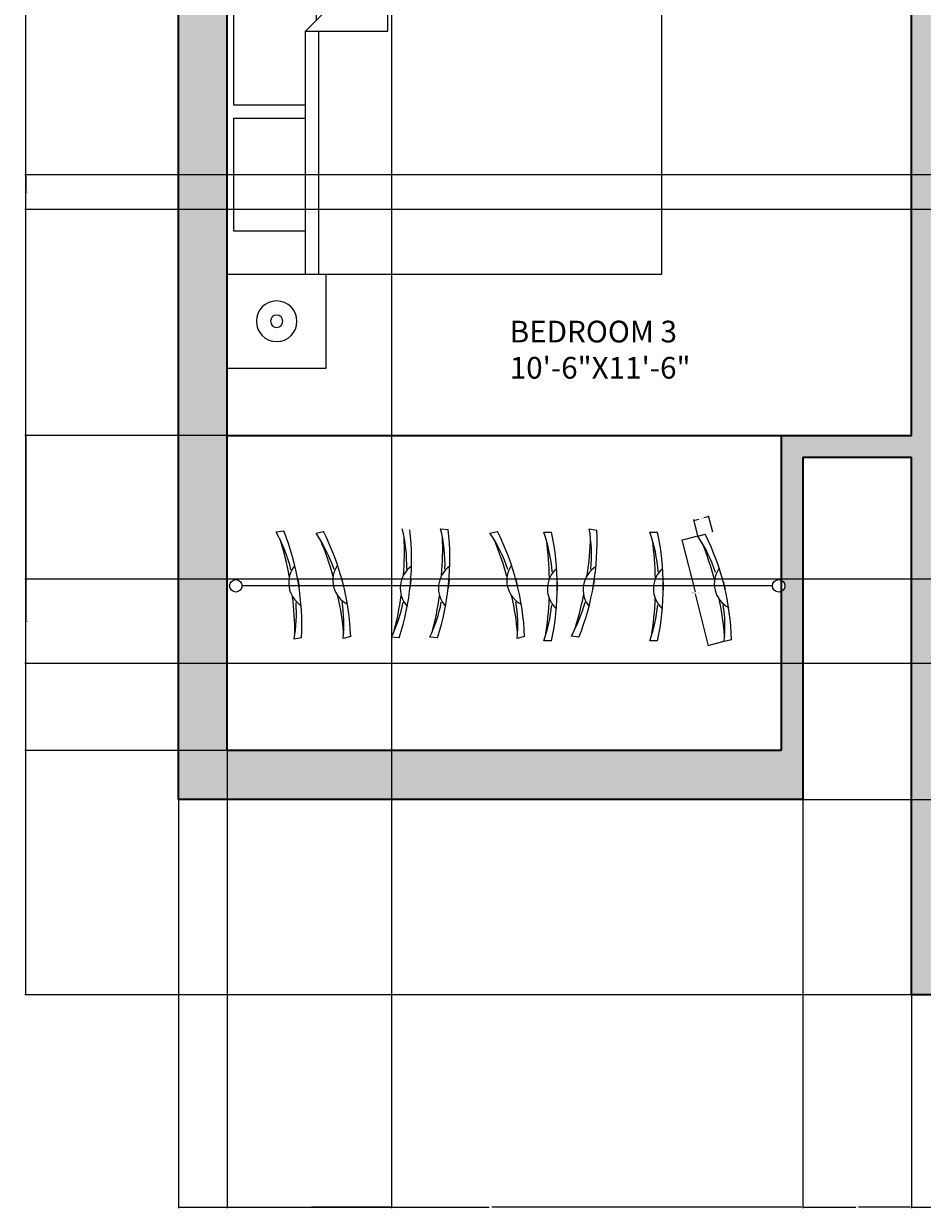
# Model space of a CAD drawing. Units: inches. Extents: x -29 to 443, y -589 to 39.
# Tile 1 of 5: x -29 to 136, y -493 to -275. Entities that reach past the tile are written whole.
import ezdxf

# ---------------------------------------------------------------- set-up
doc = ezdxf.new("R2010")
doc.units = ezdxf.units.IN
for name, color, linetype, lineweight in [('A-ANNO-DIMS', 2, 'Continuous', 18), ('A-AREA-IDEN', 7, 'Continuous', 18), ('A-FLOR-CASE', 8, 'Continuous', 18), ('A-FURN', 9, 'Continuous', 18), ('A-WALL', 7, 'Continuous', 35)]:
    doc.layers.add(name, color=color, linetype=linetype, lineweight=lineweight)
doc.layers.add('A-WALL-PATT', color=251, linetype='Continuous', lineweight=13, true_color=0x636466)
doc.styles.get("Standard").update_dxf_attribs({"font": 'arial.ttf'})
doc.dimstyles.get("Standard").update_dxf_attribs({"dimtxt": 0.18, "dimasz": 0.18, "dimexe": 0.18, "dimexo": 0.0625, "dimgap": 0.09, "dimtad": 0, "dimtih": 1, "dimtoh": 1, "dimdec": 4, "dimzin": 0, "dimdsep": 46, "dimtxsty": 'Standard', "dimcen": 0.09, "dimadec": 0, "dimazin": 0, "dimtfac": 1, "dimtdec": 4, "dimtofl": 0, "dimtmove": 0, "dimatfit": 3, "dimfxl": 1, "dimtolj": 1, "dimtzin": 0, "dimarcsym": 0})

# ---------------------------------------------------------------- blocks, each defined once
blk = doc.blocks.new('Bed - Queen')
for p, q in [((0, -80.00003), (0, 0)), ((0, 0), (59.99999, 0)), ((59.99999, 0), (59.99999, -80.00003)), ((7.99999, -1.2), (28.79998, -1.2)), ((7.99999, -14.4), (7.99999, -1.2)), ((28.79998, -1.2), (28.79998, -14.4)), ((31.19999, -1.2), (51.99999, -1.2)), ((31.19999, -14.4), (31.19999, -1.2)), ((51.99999, -1.2), (51.99999, -16.4)), ((0, -14.4), (44.8, -14.4)), ((59.99999, -29.6), (44.8, -14.4)), ((44.8, -14.4), (44.8, -29.6)), ((44.8, -16.8), (0, -16.8)), ((51.99999, -16.4), (46.79936, -16.4)), ((44.8, -29.6), (59.99999, -29.6)), ((59.99999, -80.00003), (0, -80.00003))]:
    blk.add_line(p, q)
blk = doc.blocks.new('NIGHTSTAND-SMALL')
blk.add_lwpolyline([(18.21, 17.2), (18.21, 0), (0, 0), (0, 17.2)], close=True)
for radius in [3.74, 1.13]:
    blk.add_circle((9.11, 8.6), radius)
blk = doc.blocks.new('CLOSET-HANGER')
for p, q in [((0, 20), (1.41, 20)), ((2.48, 10.82), (2.48, 9.31)), ((1.41, 0), (0, 0))]:
    blk.add_line(p, q)
for centre, radius, start, end in [((-25.67, 10.78), 27.27, 4.0274, 19.7451), ((-44.73, 10), 47.21, 347.7725, 12.2275), ((-51.84, 10.97), 52.87, 0.586, 8.2931), ((5.62, 9.59), 4.96, 130.682, 228.431), ((-25.8, 9.2), 27.39, 340.3791, 354.5177), ((-51.82, 9.48), 52.84, 350.6368, 358.15)]:
    blk.add_arc(centre, radius, start, end)
blk = doc.blocks.new('*D16')
at = {"layer": 'A-ANNO-DIMS', "color": 0, "lineweight": -2, "transparency": 16777216}
for p, q in [((95.05, -369.15), (92.03, -369.91)), ((92.24, -370.04), (94.58, -379.38)), ((97, -389.09), (94.67, -379.75)), ((99.9, -388.55), (96.87, -389.31))]:
    blk.add_line(p, q, dxfattribs=at)
at = {"layer": 'A-ANNO-DIMS', "color": 0, "transparency": 16777216}
for points in [[(92.27, -370.03), (92.21, -370.05), (92.2, -369.86)], [(97.03, -389.08), (96.97, -389.1), (97.05, -389.26)]]:
    blk.add_solid(points, dxfattribs=at)
at = {"layer": 'Defpoints', "color": 0, "transparency": 16777216}
for p in [(92.2, -369.86), (95.11, -369.14), (99.96, -388.54)]:
    blk.add_point(p, dxfattribs=at)
at = {"layer": 'A-ANNO-DIMS', "color": 0, "transparency": 16777216, "insert": (94.62, -379.56), "char_height": 0.18, "attachment_point": 5}
blk.add_mtext('\\A1;HANGER 20 TYP.', dxfattribs=at)
blk = doc.blocks.new('*D17')
at = {"layer": 'A-ANNO-DIMS', "color": 0, "lineweight": -2, "transparency": 16777216}
for p, q in [((95.09, -369.08), (94.34, -366.05)), ((94.56, -366.18), (95.3, -366)), ((96.96, -365.58), (96.22, -365.77)), ((97.85, -368.39), (97.09, -365.37))]:
    blk.add_line(p, q, dxfattribs=at)
at = {"layer": 'A-ANNO-DIMS', "color": 0, "transparency": 16777216}
for points in [[(94.55, -366.15), (94.57, -366.21), (94.38, -366.23)], [(96.95, -365.55), (96.97, -365.61), (97.14, -365.54)]]:
    blk.add_solid(points, dxfattribs=at)
at = {"layer": 'Defpoints', "color": 0, "transparency": 16777216}
for p in [(97.14, -365.54), (97.86, -368.45), (95.11, -369.14)]:
    blk.add_point(p, dxfattribs=at)
at = {"layer": 'A-ANNO-DIMS', "color": 0, "transparency": 16777216, "insert": (95.76, -365.88), "char_height": 0.18, "attachment_point": 5}
blk.add_mtext('\\A1;3 TYP.', dxfattribs=at)
blk = doc.blocks.new('*D37')
at = {"layer": 'A-ANNO-DIMS', "color": 0, "lineweight": -2, "transparency": 16777216}
for p, q in [((-0.63, 14.39), (-28.85, 14.39)), ((-28.67, 14.21), (-28.67, -219.43)), ((-28.67, -453.43), (-28.67, -219.8)), ((134.37, -453.61), (-28.85, -453.61))]:
    blk.add_line(p, q, dxfattribs=at)
at = {"layer": 'A-ANNO-DIMS', "color": 0, "transparency": 16777216}
for points in [[(-28.7, 14.21), (-28.64, 14.21), (-28.67, 14.39)], [(-28.7, -453.43), (-28.64, -453.43), (-28.67, -453.61)]]:
    blk.add_solid(points, dxfattribs=at)
at = {"layer": 'Defpoints', "color": 0, "transparency": 16777216}
for p in [(-0.56, 14.39), (-28.67, -453.61), (134.44, -453.61)]:
    blk.add_point(p, dxfattribs=at)
at = {"layer": 'A-ANNO-DIMS', "color": 0, "transparency": 16777216, "insert": (-28.67, -219.61), "char_height": 0.18, "attachment_point": 5}
blk.add_mtext('\\A1;468', dxfattribs=at)
blk = doc.blocks.new('*D38')
at = {"layer": 'A-ANNO-DIMS', "color": 0, "lineweight": -2, "transparency": 16777216}
for p, q in [((8.44, 5.32), (8.44, -492.89)), ((38.66, 5.51), (38.66, -492.89)), ((8.62, -492.71), (23.16, -492.71)), ((38.48, -492.71), (23.94, -492.71))]:
    blk.add_line(p, q, dxfattribs=at)
at = {"layer": 'A-ANNO-DIMS', "color": 0, "transparency": 16777216}
for points in [[(8.62, -492.68), (8.62, -492.74), (8.44, -492.71)], [(38.48, -492.68), (38.48, -492.74), (38.66, -492.71)]]:
    blk.add_solid(points, dxfattribs=at)
at = {"layer": 'Defpoints', "color": 0, "transparency": 16777216}
for p in [(8.44, 5.39), (38.66, 5.58), (8.44, -492.71)]:
    blk.add_point(p, dxfattribs=at)
at = {"layer": 'A-ANNO-DIMS', "color": 0, "transparency": 16777216, "insert": (23.55, -492.71), "char_height": 0.18, "attachment_point": 5}
blk.add_mtext('\\A1;30.23', dxfattribs=at)
blk = doc.blocks.new('*D42')
at = {"layer": 'A-ANNO-DIMS', "color": 0, "lineweight": -2, "transparency": 16777216}
for p, q in [((114.5, -417.61), (383.85, -417.61)), ((383.67, -417.79), (383.67, -435.43)), ((383.67, -453.43), (383.67, -435.8)), ((134.5, -453.61), (383.85, -453.61))]:
    blk.add_line(p, q, dxfattribs=at)
at = {"layer": 'A-ANNO-DIMS', "color": 0, "transparency": 16777216}
for points in [[(383.64, -417.79), (383.7, -417.79), (383.67, -417.61)], [(383.64, -453.43), (383.7, -453.43), (383.67, -453.61)]]:
    blk.add_solid(points, dxfattribs=at)
at = {"layer": 'Defpoints', "color": 0, "transparency": 16777216}
for p in [(114.44, -417.61), (134.44, -453.61), (383.67, -453.61)]:
    blk.add_point(p, dxfattribs=at)
at = {"layer": 'A-ANNO-DIMS', "color": 0, "transparency": 16777216, "insert": (383.67, -435.61), "char_height": 0.18, "attachment_point": 5}
blk.add_mtext('\\A1;36', dxfattribs=at)
blk = doc.blocks.new('*D46')
at = {"layer": 'A-ANNO-DIMS', "color": 0, "lineweight": -2, "transparency": 16777216}
for p, q in [((114.44, -417.68), (114.44, -492.89)), ((134.44, -453.68), (134.44, -492.89)), ((114.62, -492.71), (124.22, -492.71)), ((134.26, -492.71), (124.66, -492.71))]:
    blk.add_line(p, q, dxfattribs=at)
at = {"layer": 'A-ANNO-DIMS', "color": 0, "transparency": 16777216}
for points in [[(114.62, -492.68), (114.62, -492.74), (114.44, -492.71)], [(134.26, -492.68), (134.26, -492.74), (134.44, -492.71)]]:
    blk.add_solid(points, dxfattribs=at)
at = {"layer": 'Defpoints', "color": 0, "transparency": 16777216}
for p in [(114.44, -417.61), (134.44, -453.61), (134.44, -492.71)]:
    blk.add_point(p, dxfattribs=at)
at = {"layer": 'A-ANNO-DIMS', "color": 0, "transparency": 16777216, "insert": (124.44, -492.71), "char_height": 0.18, "attachment_point": 5}
blk.add_mtext('\\A1;20', dxfattribs=at)
blk = doc.blocks.new('*D47')
at = {"layer": 'A-ANNO-DIMS', "color": 0, "lineweight": -2, "transparency": 16777216}
for p, q in [((-0.56, -417.68), (-0.56, -492.89)), ((114.44, -417.68), (114.44, -492.89)), ((-0.38, -492.71), (56.65, -492.71)), ((114.26, -492.71), (57.22, -492.71))]:
    blk.add_line(p, q, dxfattribs=at)
at = {"layer": 'A-ANNO-DIMS', "color": 0, "transparency": 16777216}
for points in [[(-0.38, -492.68), (-0.38, -492.74), (-0.56, -492.71)], [(114.26, -492.68), (114.26, -492.74), (114.44, -492.71)]]:
    blk.add_solid(points, dxfattribs=at)
at = {"layer": 'Defpoints', "color": 0, "transparency": 16777216}
for p in [(-0.56, -417.61), (114.44, -417.61), (114.44, -492.71)]:
    blk.add_point(p, dxfattribs=at)
at = {"layer": 'A-ANNO-DIMS', "color": 0, "transparency": 16777216, "insert": (56.94, -492.71), "char_height": 0.18, "attachment_point": 5}
blk.add_mtext('\\A1;115', dxfattribs=at)
blk = doc.blocks.new('*D48')
at = {"layer": 'A-ANNO-DIMS', "color": 0, "lineweight": -2, "transparency": 16777216}
for p, q in [((110.37, -350.61), (-28.85, -350.61)), ((-28.67, -350.79), (-28.67, -379.43)), ((-28.67, -408.43), (-28.67, -379.8)), ((110.37, -408.61), (-28.85, -408.61))]:
    blk.add_line(p, q, dxfattribs=at)
at = {"layer": 'A-ANNO-DIMS', "color": 0, "transparency": 16777216}
for points in [[(-28.7, -350.79), (-28.64, -350.79), (-28.67, -350.61)], [(-28.7, -408.43), (-28.64, -408.43), (-28.67, -408.61)]]:
    blk.add_solid(points, dxfattribs=at)
at = {"layer": 'Defpoints', "color": 0, "transparency": 16777216}
for p in [(-28.67, -350.61), (110.44, -350.61), (110.44, -408.61)]:
    blk.add_point(p, dxfattribs=at)
at = {"layer": 'A-ANNO-DIMS', "color": 0, "transparency": 16777216, "insert": (-28.67, -379.61), "char_height": 0.18, "attachment_point": 5}
blk.add_mtext('\\A1;58', dxfattribs=at)
blk = doc.blocks.new('*D54')
at = {"layer": 'A-ANNO-DIMS', "color": 0, "lineweight": -2, "transparency": 16777216}
for p, q in [((134.44, -453.68), (134.44, -492.89)), ((147.44, -453.68), (147.44, -492.89)), ((134.62, -492.71), (140.73, -492.71)), ((147.26, -492.71), (141.15, -492.71))]:
    blk.add_line(p, q, dxfattribs=at)
at = {"layer": 'A-ANNO-DIMS', "color": 0, "transparency": 16777216}
for points in [[(134.62, -492.68), (134.62, -492.74), (134.44, -492.71)], [(147.26, -492.68), (147.26, -492.74), (147.44, -492.71)]]:
    blk.add_solid(points, dxfattribs=at)
at = {"layer": 'Defpoints', "color": 0, "transparency": 16777216}
for p in [(134.44, -453.61), (147.44, -453.61), (147.44, -492.71)]:
    blk.add_point(p, dxfattribs=at)
at = {"layer": 'A-ANNO-DIMS', "color": 0, "transparency": 16777216, "insert": (140.94, -492.71), "char_height": 0.18, "attachment_point": 5}
blk.add_mtext('\\A1;13', dxfattribs=at)
blk = doc.blocks.new('*D84')
at = {"layer": 'A-ANNO-DIMS', "color": 0, "lineweight": -2, "transparency": 16777216}
for p, q in [((350.37, -302.61), (-28.85, -302.61)), ((-28.67, -302.79), (-28.67, -305.61)), ((-28.67, -308.79), (-28.67, -305.97)), ((347.03, -308.97), (-28.85, -308.97))]:
    blk.add_line(p, q, dxfattribs=at)
at = {"layer": 'A-ANNO-DIMS', "color": 0, "transparency": 16777216}
for points in [[(-28.7, -302.79), (-28.64, -302.79), (-28.67, -302.61)], [(-28.7, -308.79), (-28.64, -308.79), (-28.67, -308.97)]]:
    blk.add_solid(points, dxfattribs=at)
at = {"layer": 'Defpoints', "color": 0, "transparency": 16777216}
for p in [(350.44, -302.61), (-28.67, -308.97), (347.09, -308.97)]:
    blk.add_point(p, dxfattribs=at)
at = {"layer": 'A-ANNO-DIMS', "color": 0, "transparency": 16777216, "insert": (-28.67, -305.79), "char_height": 0.18, "attachment_point": 5}
blk.add_mtext('\\A1;6.353', dxfattribs=at)
blk = doc.blocks.new('*D85')
at = {"layer": 'A-ANNO-DIMS', "color": 0, "lineweight": -2, "transparency": 16777216}
for p, q in [((346.2, -377.07), (-28.85, -377.07)), ((-28.67, -377.25), (-28.67, -384.66)), ((-28.67, -392.43), (-28.67, -385.02)), ((350.37, -392.61), (-28.85, -392.61))]:
    blk.add_line(p, q, dxfattribs=at)
at = {"layer": 'A-ANNO-DIMS', "color": 0, "transparency": 16777216}
for points in [[(-28.7, -377.25), (-28.64, -377.25), (-28.67, -377.07)], [(-28.7, -392.43), (-28.64, -392.43), (-28.67, -392.61)]]:
    blk.add_solid(points, dxfattribs=at)
at = {"layer": 'Defpoints', "color": 0, "transparency": 16777216}
for p in [(-28.67, -377.07), (346.26, -377.07), (350.44, -392.61)]:
    blk.add_point(p, dxfattribs=at)
at = {"layer": 'A-ANNO-DIMS', "color": 0, "transparency": 16777216, "insert": (-28.67, -384.84), "char_height": 0.18, "attachment_point": 5}
blk.add_mtext('\\A1;15.544', dxfattribs=at)

msp = doc.modelspace()

# ---------------------------------------------------------------- hatches: boundary and pattern name
at = {"layer": 'A-WALL-PATT'}
h = msp.add_hatch(color=256, dxfattribs=at)
h.dxf.hatch_style = 1
h.paths.add_polyline_path([(8.4359, 5.3851), (38.6638, 5.3851), (38.6638, 14.3851), (-0.5641, 14.3851), (-0.5641, -161.7206), (8.4359, -161.7206), (8.4359, -154.6149), (98.4359, -154.6149), (98.4359, -169.6149), (102.4359, -169.6149), (102.4359, -154.6149), (144.4359, -154.6149), (144.4359, -141.6149), (140.4359, -141.6149), (140.4359, -150.6149), (8.4359, -150.6149)])
h.paths.add_polyline_path([(153.762, 14.3851), (92.6638, 14.3851), (92.6638, 5.3851), (140.4359, 5.3851), (140.4359, -105.5868), (144.4359, -105.5868), (144.4359, -94.6149), (153.4359, -94.6149), (153.4359, -90.6149), (144.4359, -90.6149), (144.4359, 5.3851), (153.762, 5.3851)])
h.paths.add_polyline_path([(264.576, 14.3851), (189.762, 14.3851), (189.762, 5.3851), (204.4359, 5.3851), (204.4359, -40.0486, -0.11439146), (204.5889, -40.7086), (204.5889, -67.7086, -0.11439146), (204.4359, -68.3685), (204.4359, -90.6149), (183.4359, -90.6149), (183.4359, -94.6149), (204.4359, -94.6149), (204.4359, -108.4622), (208.4359, -108.4622), (208.4359, 5.3851), (264.576, 5.3851)])
h.paths.add_polyline_path([(359.4359, 14.3851), (318.576, 14.3851), (318.576, 5.3851), (350.4359, 5.3851), (350.4359, -150.6149), (208.4359, -150.6149), (208.4359, -144.6149), (204.4359, -144.6149), (204.4359, -154.6149), (286.4359, -154.6149), (286.4359, -169.4775), (290.4359, -169.4775), (290.4359, -154.6149), (359.4359, -154.6149)])
h.paths.add_polyline_path([(8.4359, -212.6149), (98.4359, -212.6149), (102.4359, -212.6149), (102.4359, -199.6149), (98.4359, -199.6149), (98.4359, -208.6149), (8.4359, -208.6149), (8.4359, -197.7206), (-0.5641, -197.7206), (-0.5641, -417.6149), (114.4359, -417.6149), (114.4359, -354.6149), (134.4359, -354.6149), (134.4359, -453.6149), (147.4359, -453.6149), (147.4359, -444.6149), (138.4359, -444.6149), (138.4359, -212.6149), (129.4359, -212.6149), (129.4359, -216.6149), (134.4359, -216.6149), (134.4359, -350.6149), (110.4359, -350.6149), (110.4359, -377.2063, -0.30395766), (111.1497, -378.2719, -0.30395766), (110.4359, -379.3376), (110.4359, -408.6149), (8.4359, -408.6149)])
h.paths.add_polyline_path([(265.0252, -444.6149), (230.4359, -444.6149), (230.4359, -396.6149), (246.223, -396.6149), (246.223, -392.6149), (230.4359, -392.6149), (230.4359, -302.6149), (245.4886, -302.6149), (245.4886, -298.6149), (226.4359, -298.6149), (226.4359, -444.6149), (189.4359, -444.6149), (189.4359, -453.6149), (226.4359, -453.6149), (265.0252, -453.6149)])
h.paths.add_polyline_path([(359.4359, -417.6149), (359.4359, -377.3771), (350.4359, -377.3771), (350.4359, -392.6149), (276.3235, -392.6149), (276.3235, -396.6149), (350.4359, -396.6149), (350.4359, -408.6149), (350.4359, -444.6149), (319.0252, -444.6149), (319.0252, -453.6149), (359.4359, -453.6149)])
h.paths.add_polyline_path([(359.4359, -298.6149), (290.4359, -298.6149), (290.4359, -289.6207), (286.4359, -289.6207), (286.4359, -298.6149), (277.8355, -298.6149), (277.8355, -302.6149), (350.4359, -302.6149), (350.4359, -323.3771), (359.4359, -323.3771)])
h.paths.add_polyline_path([(290.4359, -226.7916), (286.4359, -226.7916), (286.4359, -253.468), (290.4359, -253.468)])

# ---------------------------------------------------------------- linework, layer by layer
at = {"layer": 'A-FLOR-CASE'}
msp.add_line((108.8451, -378.2885), (11.1271, -378.2885), dxfattribs=at)
for centre in [(10.0136, -378.2719), (109.9973, -378.2719)]:
    msp.add_circle(centre, 1.1524, dxfattribs=at)
at = {"layer": 'A-FURN'}
for p, q in [((42.2396, -377.1753), (42.0915, -378.6789)), ((40.1179, -387.8399), (38.7157, -387.7018))]:
    msp.add_line(p, q, dxfattribs=at)
for centre, radius, start, end in [((-4.8169, -373.367), 47.208, 342.146968, 6.602004), ((14.2251, -374.4549), 27.2748, 358.401871, 14.119601), ((-11.8003, -371.7039), 52.8739, 354.960525, 2.667625), ((45.2498, -378.7105), 4.9606, 125.05649, 222.805441), ((13.9423, -376.0198), 27.3896, 334.753545, 348.892145), ((-11.9296, -373.1867), 52.8401, 345.011307, 352.524443)]:
    msp.add_arc(centre, radius, start, end, dxfattribs=at)
at = {"layer": 'A-WALL'}
for p, q in [((-0.5641, -417.6149), (-0.5641, 14.3851)), ((8.4359, -408.6149), (8.4359, -212.6149)), ((134.4359, -350.6149), (134.4359, -216.6149)), ((8.4359, -350.6149), (134.4359, -350.6149)), ((110.4359, -350.6149), (110.4359, -408.6149)), ((114.4359, -354.6149), (114.4359, -417.6149)), ((114.4359, -354.6149), (134.4359, -354.6149)), ((134.4359, -453.6149), (134.4359, -354.6149)), ((110.4359, -408.6149), (8.4359, -408.6149)), ((114.4359, -417.6149), (-0.5641, -417.6149)), ((147.4359, -453.6149), (134.4359, -453.6149))]:
    msp.add_line(p, q, dxfattribs=at)

# ---------------------------------------------------------------- block references
at = {"layer": 'A-FURN'}
for name, p, rotation in [('Bed - Queen', (8.4359, -320.9746), 90), ('CLOSET-HANGER', (20.7428, -388.0921), 9.453816115787394), ('CLOSET-HANGER', (29.8103, -387.9607), 14.5215371830677), ('CLOSET-HANGER', (45.7603, -387.7013), 354.3744866708974), ('CLOSET-HANGER', (61.8318, -387.9607), 14.52153718384618), ('CLOSET-HANGER', (71.8123, -387.5212), 350.5462235724349), ('CLOSET-HANGER', (99.9555, -388.5376), 14.02384461538142)]:
    msp.add_blockref(name, p, dxfattribs=dict(at, rotation=rotation))
at = {"layer": 'A-FURN', "extrusion": (0, 0, -1), "zscale": -1}
msp.add_blockref('NIGHTSTAND-SMALL', (-26.6499, -338.1702), dxfattribs=at)
at = {"layer": 'A-FURN'}
for p in [(66.7362, -388.403), (86.259, -388.403)]:
    msp.add_blockref('CLOSET-HANGER', p, dxfattribs=at)

# ---------------------------------------------------------------- texts
at = {"layer": 'A-AREA-IDEN', "insert": (60.4633, -329.4633), "char_height": 4, "attachment_point": 1}
msp.add_mtext_dynamic_manual_height_columns('BEDROOM 3\\P10\'-6"X11\'-6"', width=60.26419, gutter_width=12.5, heights=[0], dxfattribs=at)

# ---------------------------------------------------------------- dimensions: what is measured, and where the dimension line sits
at = {"layer": 'A-ANNO-DIMS'}
for base, p1, p2, override, picture, middle in [((-28.6698, -453.6149), (-0.5641, 14.3851), (134.4359, -453.6149), {"dimdec": 0, "dimlfac": 1, "dimrnd": 0, "dimzin": 0, "dimdsep": 46, "dimlunit": 2}, '*D37', (-28.6698, -219.6149)), ((-28.6698, -308.9679), (350.4359, -302.6149), (347.093, -308.9679), {"dimdec": 3, "dimlfac": 1, "dimrnd": 0, "dimzin": 0, "dimdsep": 46, "dimlunit": 2}, '*D84', (-28.6698, -305.7914)), ((-28.6698, -350.6149), (110.4359, -408.6149), (110.4359, -350.6149), {"dimdec": 0, "dimlfac": 1, "dimrnd": 0, "dimzin": 0, "dimdsep": 46, "dimlunit": 2}, '*D48', (-28.6698, -379.6149)), ((-28.6698, -377.0712), (350.4359, -392.6149), (346.2626, -377.0712), {"dimdec": 3, "dimlfac": 1, "dimrnd": 0, "dimzin": 0, "dimdsep": 46, "dimlunit": 2}, '*D85', (-28.6698, -384.8431)), ((383.6659, -453.6149), (114.4359, -417.6149), (134.4359, -453.6149), {"dimdec": 0, "dimlfac": 1, "dimrnd": 0, "dimzin": 0, "dimdsep": 46, "dimlunit": 2}, '*D42', (383.6659, -435.6149))]:
    dim = msp.add_linear_dim(base=base, p1=p1, p2=p2, angle=90, dimstyle='Standard', override=override, dxfattribs=at)
    dim.commit()
    dim.dimension.update_dxf_attribs({"geometry": picture, "text_midpoint": middle})
for base, p1, p2, override, picture, middle in [((8.4359, -492.7145), (38.6638, 5.5764), (8.4359, 5.3851), {"dimdec": 2, "dimlfac": 1, "dimrnd": 0, "dimzin": 0, "dimdsep": 46, "dimlunit": 2}, '*D38', (23.5499, -492.7145)), ((114.4359, -492.7145), (-0.5641, -417.6149), (114.4359, -417.6149), {"dimdec": 0, "dimlfac": 1, "dimrnd": 0, "dimzin": 0, "dimdsep": 46, "dimlunit": 2}, '*D47', (56.9359, -492.7145)), ((134.4359, -492.7145), (114.4359, -417.6149), (134.4359, -453.6149), {"dimdec": 0, "dimlfac": 1, "dimrnd": 0, "dimzin": 0, "dimdsep": 46, "dimlunit": 2}, '*D46', (124.4359, -492.7145)), ((147.4359, -492.7145), (134.4359, -453.6149), (147.4359, -453.6149), {"dimdec": 0, "dimlfac": 1, "dimrnd": 0, "dimzin": 0, "dimdsep": 46, "dimlunit": 2}, '*D54', (140.9359, -492.7145))]:
    dim = msp.add_linear_dim(base=base, p1=p1, p2=p2, dimstyle='Standard', override=override, dxfattribs=at)
    dim.commit()
    dim.dimension.update_dxf_attribs({"geometry": picture, "text_midpoint": middle})
for base, p1, p2, angle, text, picture, middle in [((97.1355, -365.5397), (95.11, -369.1373), (97.8624, -368.4498), 14.023845, '<> TYP.', '*D17', (95.7594, -365.8834)), ((92.1999, -369.8641), (99.9558, -388.538), (95.11, -369.1373), 104.023845, 'HANGER <> TYP.', '*D16', (94.6228, -379.5645))]:
    dim = msp.add_linear_dim(base=base, p1=p1, p2=p2, angle=angle, text=text, dimstyle='Standard', override={"dimdec": 0, "dimlfac": 1, "dimrnd": 0, "dimzin": 0, "dimdsep": 46, "dimlunit": 2}, dxfattribs=at)
    dim.commit()
    dim.dimension.update_dxf_attribs({"geometry": picture, "text_midpoint": middle})

doc.saveas('drawing.dxf')
